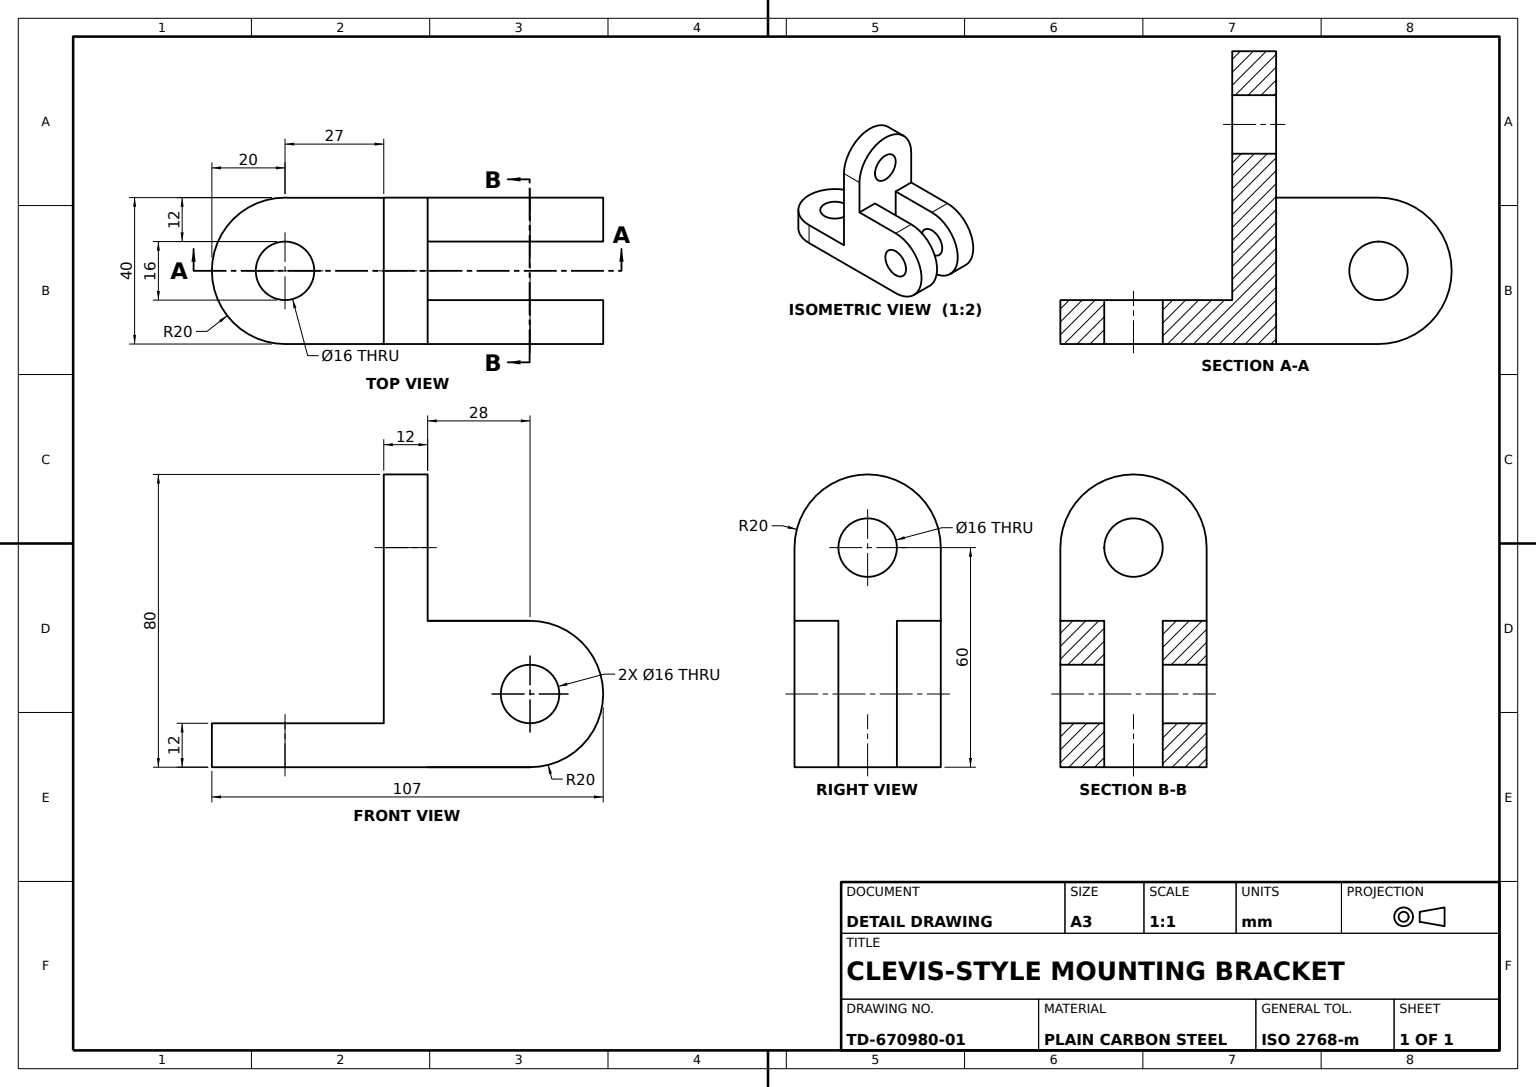
from build123d import *

# Parameters (mm, degrees)
UPRIGHT_LUG_SKETCH_R     = 8
UPRIGHT_LUG_DEPTH        = 12
CLEVIS_SIDE_LUG_SKETCH_R = 8
CLEVIS_SIDE_LUG_DEPTH    = 12
HORIZONTAL_LUG_SKETCH_R  = 8
HORIZONTAL_LUG_DEPTH     = 12


with BuildPart() as part:
    # Upright Lug Sketch → Upright Lug (new body)
    with BuildSketch(Plane.XY):
        with BuildLine():
            Line((-20, 0), (20, 0))
            Line((20, 0), (20, 60))
            ThreePointArc((20, 60), (0, 80), (-20, 60))
            Line((-20, 60), (-20, 0))
        make_face()
        with Locations((0, 60)):
            Circle(UPRIGHT_LUG_SKETCH_R, mode=Mode.SUBTRACT)
    extrude(amount=UPRIGHT_LUG_DEPTH)

    # Clevis Side Lug Sketch → Clevis Side Lug (add)
    with BuildSketch(Plane(origin=(20, 0, 0), x_dir=(0, 0, -1), z_dir=(1, 0, 0))):
        with BuildLine():
            Line((0, 0), (-40, 0))
            ThreePointArc((-40, 0), (-60, 20), (-40, 40))
            Line((-40, 40), (0, 40))
            Line((0, 40), (0, 0))
        make_face()
        with Locations(Location((-40, 20, 0), (0, 0, 90))):
            Circle(CLEVIS_SIDE_LUG_SKETCH_R, mode=Mode.SUBTRACT)
    clevis_side_lug = extrude(amount=-CLEVIS_SIDE_LUG_DEPTH)

    # Clevis Side Lug Mirror: Clevis Side Lug across plane
    add(clevis_side_lug.mirror(Plane(origin=(0, 0, 0), x_dir=(0, 0, 1), z_dir=(1, 0, 0))))

    # Horizontal Lug Sketch → Horizontal Lug (add)
    with BuildSketch(Plane.XZ):
        with BuildLine():
            Line((-20, 12), (19.961751116, 12))
            Line((19.961751116, 12), (19.961751116, -25.763677886))
            ThreePointArc((19.961751116, -25.763677886), (0.618456819, -46.990435492), (-20, -27))
            Line((-20, -27), (-20, 12))
        make_face()
        with Locations((0, -27)):
            Circle(HORIZONTAL_LUG_SKETCH_R, mode=Mode.SUBTRACT)
    extrude(amount=-HORIZONTAL_LUG_DEPTH)


solid = part.part
